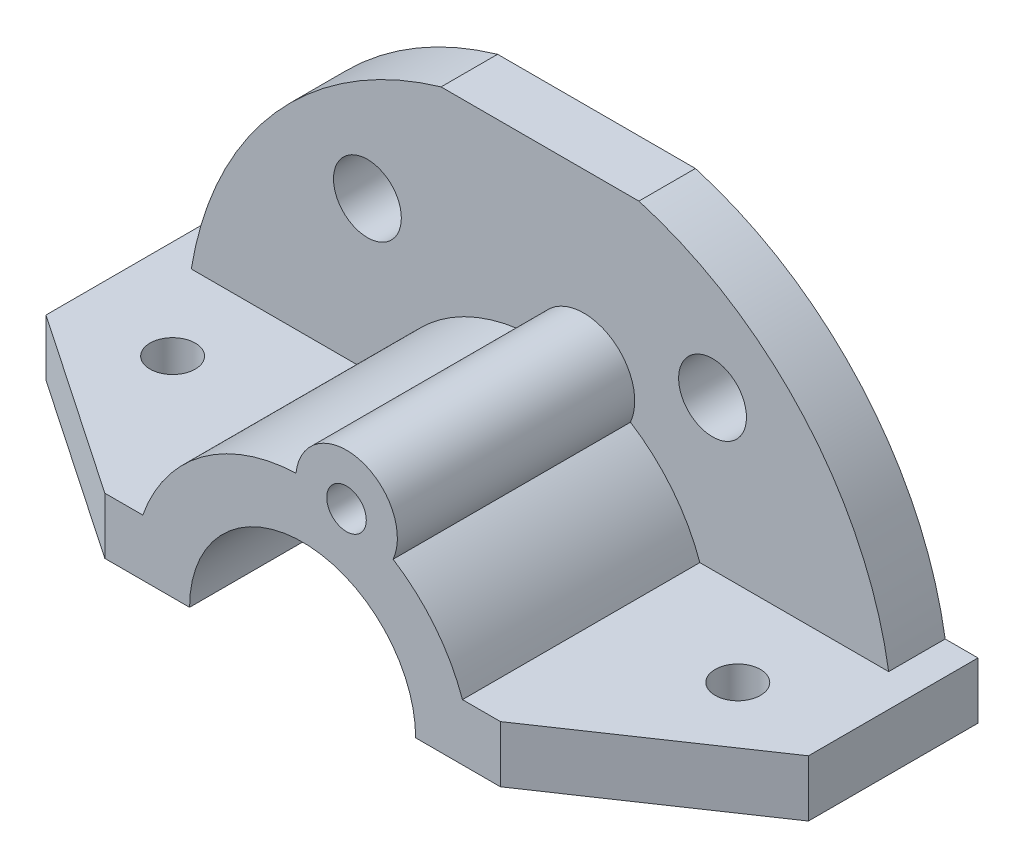
ISO-10303-21;
HEADER;
FILE_DESCRIPTION(('STEP AP214'),'2;1');
FILE_NAME('part.step','',(''),(''),'','','');
FILE_SCHEMA(('AUTOMOTIVE_DESIGN { 1 0 10303 214 1 1 1 1 }'));
ENDSEC;
DATA;
#1=APPLICATION_CONTEXT('core data for automotive mechanical design processes');
#2=APPLICATION_PROTOCOL_DEFINITION('international standard','automotive_design',2000,#1);
#3=PRODUCT_CONTEXT('',#1,'mechanical');
#4=PRODUCT('Part','Part','',(#3));
#5=PRODUCT_RELATED_PRODUCT_CATEGORY('part','',(#4));
#6=PRODUCT_DEFINITION_FORMATION('','',#4);
#7=PRODUCT_DEFINITION_CONTEXT('part definition',#1,'design');
#8=PRODUCT_DEFINITION('design','',#6,#7);
#9=PRODUCT_DEFINITION_SHAPE('','',#8);
#10=(LENGTH_UNIT() NAMED_UNIT(*) SI_UNIT(.MILLI.,.METRE.));
#11=(NAMED_UNIT(*) PLANE_ANGLE_UNIT() SI_UNIT($,.RADIAN.));
#12=(NAMED_UNIT(*) SI_UNIT($,.STERADIAN.) SOLID_ANGLE_UNIT());
#13=UNCERTAINTY_MEASURE_WITH_UNIT(LENGTH_MEASURE(1.E-05),#10,'distance_accuracy_value','');
#14=(GEOMETRIC_REPRESENTATION_CONTEXT(3) GLOBAL_UNCERTAINTY_ASSIGNED_CONTEXT((#13)) GLOBAL_UNIT_ASSIGNED_CONTEXT((#10,
#11,#12)) REPRESENTATION_CONTEXT('',''));
#15=CARTESIAN_POINT('',(0.,0.,0.));
#16=DIRECTION('',(0.,0.,1.));
#17=DIRECTION('',(1.,0.,0.));
#18=AXIS2_PLACEMENT_3D('',#15,#16,#17);
#19=CARTESIAN_POINT('',(0.,0.,52.));
#20=DIRECTION('',(0.,0.,-1.));
#21=DIRECTION('',(-1.,0.,0.));
#22=AXIS2_PLACEMENT_3D('',#19,#20,#21);
#23=CYLINDRICAL_SURFACE('',#22,30.);
#24=CARTESIAN_POINT('',(0.,0.,10.));
#25=DIRECTION('',(0.,0.,1.));
#26=DIRECTION('',(1.,0.,0.));
#27=AXIS2_PLACEMENT_3D('',#24,#25,#26);
#28=CIRCLE('',#27,30.);
#29=CARTESIAN_POINT('',(28.2842712474618,10.0000000000002,10.));
#30=VERTEX_POINT('',#29);
#31=CARTESIAN_POINT('',(16.0101416866023,25.370758033116,10.));
#32=VERTEX_POINT('',#31);
#33=EDGE_CURVE('E176',#30,#32,#28,.T.);
#34=ORIENTED_EDGE('',*,*,#33,.T.);
#35=DIRECTION('',(0.,0.,1.));
#36=VECTOR('',#35,1.);
#37=CARTESIAN_POINT('',(16.0101416866023,25.370758033116,27.));
#38=LINE('',#37,#36);
#39=CARTESIAN_POINT('',(16.0101416866023,25.370758033116,52.));
#40=VERTEX_POINT('',#39);
#41=EDGE_CURVE('E11',#32,#40,#38,.T.);
#42=ORIENTED_EDGE('',*,*,#41,.T.);
#43=CARTESIAN_POINT('',(0.,0.,52.));
#44=DIRECTION('',(0.,0.,1.));
#45=DIRECTION('',(1.,0.,0.));
#46=AXIS2_PLACEMENT_3D('',#43,#44,#45);
#47=CIRCLE('',#46,30.);
#48=CARTESIAN_POINT('',(28.2842712474618,10.0000000000002,52.));
#49=VERTEX_POINT('',#48);
#50=EDGE_CURVE('E172',#49,#40,#47,.T.);
#51=ORIENTED_EDGE('',*,*,#50,.F.);
#52=DIRECTION('',(0.,0.,-1.));
#53=VECTOR('',#52,1.);
#54=CARTESIAN_POINT('',(28.2842712474618,10.0000000000002,52.));
#55=LINE('',#54,#53);
#56=EDGE_CURVE('E202',#49,#30,#55,.T.);
#57=ORIENTED_EDGE('',*,*,#56,.T.);
#58=EDGE_LOOP('',(#34,#42,#51,#57));
#59=FACE_BOUND('',#58,.T.);
#60=ADVANCED_FACE('F43',(#59),#23,.T.);
#61=CARTESIAN_POINT('',(0.,0.,10.));
#62=DIRECTION('',(0.,1.,0.));
#63=DIRECTION('',(-1.,0.,0.));
#64=AXIS2_PLACEMENT_3D('',#61,#62,#63);
#65=PLANE('',#64);
#66=CARTESIAN_POINT('',(-50.,-1.73472347597681E-13,25.));
#67=DIRECTION('',(0.,1.,0.));
#68=DIRECTION('',(-1.,0.,0.));
#69=AXIS2_PLACEMENT_3D('',#66,#67,#68);
#70=CIRCLE('',#69,4.00000000000001);
#71=CARTESIAN_POINT('',(-54.,-1.87438272953053E-13,25.));
#72=VERTEX_POINT('',#71);
#73=EDGE_CURVE('E328',#72,#72,#70,.T.);
#74=ORIENTED_EDGE('',*,*,#73,.T.);
#75=EDGE_LOOP('',(#74));
#76=FACE_BOUND('',#75,.T.);
#77=DIRECTION('',(0.826972369841966,0.,0.562242562883638));
#78=VECTOR('',#77,1.);
#79=CARTESIAN_POINT('',(-35.2419558451316,2.18575157973078E-13,51.8354988879526));
#80=LINE('',#79,#78);
#81=CARTESIAN_POINT('',(-67.5,2.18575157973078E-13,29.9038768886436));
#82=VERTEX_POINT('',#81);
#83=CARTESIAN_POINT('',(-35.,2.18575157973078E-13,52.));
#84=VERTEX_POINT('',#83);
#85=EDGE_CURVE('E265',#82,#84,#80,.T.);
#86=ORIENTED_EDGE('',*,*,#85,.F.);
#87=DIRECTION('',(0.,0.,1.));
#88=VECTOR('',#87,1.);
#89=CARTESIAN_POINT('',(-67.5,2.18575157973078E-13,52.));
#90=LINE('',#89,#88);
#91=CARTESIAN_POINT('',(-67.5,2.18575157973078E-13,-0.0961231113559209));
#92=VERTEX_POINT('',#91);
#93=EDGE_CURVE('E303',#92,#82,#90,.T.);
#94=ORIENTED_EDGE('',*,*,#93,.F.);
#95=DIRECTION('',(-0.999880138885791,0.,-0.015482501791758));
#96=VECTOR('',#95,1.);
#97=CARTESIAN_POINT('',(-67.5,2.18575157973078E-13,-0.0961231113559209));
#98=LINE('',#97,#96);
#99=CARTESIAN_POINT('',(-61.6948133962651,2.18575157973078E-13,-0.00623352509614107));
#100=VERTEX_POINT('',#99);
#101=EDGE_CURVE('E296',#100,#92,#98,.T.);
#102=ORIENTED_EDGE('',*,*,#101,.F.);
#103=DIRECTION('',(0.,0.,-1.));
#104=VECTOR('',#103,1.);
#105=CARTESIAN_POINT('',(-61.6948133962651,2.18575157973078E-13,-0.00623352509614107));
#106=LINE('',#105,#104);
#107=CARTESIAN_POINT('',(-61.6948133962651,-2.15406289676469E-13,0.));
#108=VERTEX_POINT('',#107);
#109=EDGE_CURVE('E315',#108,#100,#106,.T.);
#110=ORIENTED_EDGE('',*,*,#109,.F.);
#111=DIRECTION('',(1.,0.,0.));
#112=VECTOR('',#111,1.);
#113=CARTESIAN_POINT('',(0.,0.,0.));
#114=LINE('',#113,#112);
#115=CARTESIAN_POINT('',(-20.,0.,0.));
#116=VERTEX_POINT('',#115);
#117=EDGE_CURVE('E216',#108,#116,#114,.T.);
#118=ORIENTED_EDGE('',*,*,#117,.T.);
#119=DIRECTION('',(0.,0.,1.));
#120=VECTOR('',#119,1.);
#121=CARTESIAN_POINT('',(-20.,0.,-125.));
#122=LINE('',#121,#120);
#123=CARTESIAN_POINT('',(-20.,0.,52.));
#124=VERTEX_POINT('',#123);
#125=EDGE_CURVE('E200',#116,#124,#122,.T.);
#126=ORIENTED_EDGE('',*,*,#125,.T.);
#127=DIRECTION('',(1.,0.,0.));
#128=VECTOR('',#127,1.);
#129=CARTESIAN_POINT('',(0.,0.,52.));
#130=LINE('',#129,#128);
#131=EDGE_CURVE('E188',#84,#124,#130,.T.);
#132=ORIENTED_EDGE('',*,*,#131,.F.);
#133=EDGE_LOOP('',(#86,#94,#102,#110,#118,#126,#132));
#134=FACE_BOUND('',#133,.T.);
#135=ADVANCED_FACE('F44',(#76,#134),#65,.F.);
#136=CARTESIAN_POINT('',(50.,1.73472347597681E-13,25.));
#137=DIRECTION('',(0.,1.,0.));
#138=DIRECTION('',(-1.,0.,0.));
#139=AXIS2_PLACEMENT_3D('',#136,#137,#138);
#140=CIRCLE('',#139,4.00000000000001);
#141=CARTESIAN_POINT('',(46.,1.59506422242308E-13,25.));
#142=VERTEX_POINT('',#141);
#143=EDGE_CURVE('E316',#142,#142,#140,.T.);
#144=ORIENTED_EDGE('',*,*,#143,.T.);
#145=EDGE_LOOP('',(#144));
#146=FACE_BOUND('',#145,.T.);
#147=DIRECTION('',(0.828109472135937,0.,-0.560566411907403));
#148=VECTOR('',#147,1.);
#149=CARTESIAN_POINT('',(35.1371530595682,2.18575157973078E-13,51.9071579289076));
#150=LINE('',#149,#148);
#151=CARTESIAN_POINT('',(35.,2.18575157973078E-13,52.));
#152=VERTEX_POINT('',#151);
#153=CARTESIAN_POINT('',(67.5,2.18575157973078E-13,30.));
#154=VERTEX_POINT('',#153);
#155=EDGE_CURVE('E70',#152,#154,#150,.T.);
#156=ORIENTED_EDGE('',*,*,#155,.F.);
#157=CARTESIAN_POINT('',(20.,0.,52.));
#158=VERTEX_POINT('',#157);
#159=EDGE_CURVE('E184',#158,#152,#130,.T.);
#160=ORIENTED_EDGE('',*,*,#159,.F.);
#161=DIRECTION('',(0.,0.,1.));
#162=VECTOR('',#161,1.);
#163=CARTESIAN_POINT('',(20.,0.,-125.));
#164=LINE('',#163,#162);
#165=CARTESIAN_POINT('',(20.,0.,0.));
#166=VERTEX_POINT('',#165);
#167=EDGE_CURVE('E271',#158,#166,#164,.F.);
#168=ORIENTED_EDGE('',*,*,#167,.T.);
#169=CARTESIAN_POINT('',(67.5,2.18575157973078E-13,0.));
#170=VERTEX_POINT('',#169);
#171=EDGE_CURVE('E204',#166,#170,#114,.T.);
#172=ORIENTED_EDGE('',*,*,#171,.T.);
#173=DIRECTION('',(0.,0.,-1.));
#174=VECTOR('',#173,1.);
#175=CARTESIAN_POINT('',(67.5,2.18575157973078E-13,52.));
#176=LINE('',#175,#174);
#177=EDGE_CURVE('E283',#154,#170,#176,.T.);
#178=ORIENTED_EDGE('',*,*,#177,.F.);
#179=EDGE_LOOP('',(#156,#160,#168,#172,#178));
#180=FACE_BOUND('',#179,.T.);
#181=ADVANCED_FACE('F367',(#146,#180),#65,.F.);
#182=CARTESIAN_POINT('',(0.,10.0000000000002,52.));
#183=DIRECTION('',(0.,-1.,0.));
#184=DIRECTION('',(0.,0.,-1.));
#185=AXIS2_PLACEMENT_3D('',#182,#183,#184);
#186=PLANE('',#185);
#187=CARTESIAN_POINT('',(50.,10.0000000000002,25.));
#188=DIRECTION('',(0.,1.,0.));
#189=DIRECTION('',(0.,0.,1.));
#190=AXIS2_PLACEMENT_3D('',#187,#188,#189);
#191=CIRCLE('',#190,4.00000000000001);
#192=CARTESIAN_POINT('',(50.,10.0000000000002,29.));
#193=VERTEX_POINT('',#192);
#194=EDGE_CURVE('E335',#193,#193,#191,.T.);
#195=ORIENTED_EDGE('',*,*,#194,.F.);
#196=EDGE_LOOP('',(#195));
#197=FACE_BOUND('',#196,.T.);
#198=DIRECTION('',(0.828109472135937,0.,-0.560566411907403));
#199=VECTOR('',#198,1.);
#200=CARTESIAN_POINT('',(35.1371530595682,10.0000000000002,51.9071579289076));
#201=LINE('',#200,#199);
#202=CARTESIAN_POINT('',(35.,10.0000000000002,52.));
#203=VERTEX_POINT('',#202);
#204=CARTESIAN_POINT('',(67.5,10.0000000000002,30.));
#205=VERTEX_POINT('',#204);
#206=EDGE_CURVE('E320',#203,#205,#201,.T.);
#207=ORIENTED_EDGE('',*,*,#206,.T.);
#208=DIRECTION('',(0.,0.,-1.));
#209=VECTOR('',#208,1.);
#210=CARTESIAN_POINT('',(67.5,10.0000000000002,52.));
#211=LINE('',#210,#209);
#212=CARTESIAN_POINT('',(67.5,10.0000000000002,0.));
#213=VERTEX_POINT('',#212);
#214=EDGE_CURVE('E288',#205,#213,#211,.T.);
#215=ORIENTED_EDGE('',*,*,#214,.T.);
#216=DIRECTION('',(-1.,0.,0.));
#217=VECTOR('',#216,1.);
#218=CARTESIAN_POINT('',(61.6948133962653,10.0000000000002,0.));
#219=LINE('',#218,#217);
#220=CARTESIAN_POINT('',(61.6948133962653,10.0000000000002,0.));
#221=VERTEX_POINT('',#220);
#222=EDGE_CURVE('E290',#213,#221,#219,.T.);
#223=ORIENTED_EDGE('',*,*,#222,.T.);
#224=DIRECTION('',(0.,0.,1.));
#225=VECTOR('',#224,1.);
#226=CARTESIAN_POINT('',(61.6948133962653,10.0000000000002,52.));
#227=LINE('',#226,#225);
#228=CARTESIAN_POINT('',(61.6948133962653,10.0000000000002,10.));
#229=VERTEX_POINT('',#228);
#230=EDGE_CURVE('E284',#221,#229,#227,.T.);
#231=ORIENTED_EDGE('',*,*,#230,.T.);
#232=DIRECTION('',(-1.,0.,0.));
#233=VECTOR('',#232,1.);
#234=CARTESIAN_POINT('',(0.,10.0000000000002,10.));
#235=LINE('',#234,#233);
#236=EDGE_CURVE('E194',#229,#30,#235,.T.);
#237=ORIENTED_EDGE('',*,*,#236,.T.);
#238=ORIENTED_EDGE('',*,*,#56,.F.);
#239=DIRECTION('',(-1.,0.,0.));
#240=VECTOR('',#239,1.);
#241=CARTESIAN_POINT('',(0.,10.0000000000002,52.));
#242=LINE('',#241,#240);
#243=EDGE_CURVE('E179',#203,#49,#242,.T.);
#244=ORIENTED_EDGE('',*,*,#243,.F.);
#245=EDGE_LOOP('',(#207,#215,#223,#231,#237,#238,#244));
#246=FACE_BOUND('',#245,.T.);
#247=ADVANCED_FACE('F407',(#197,#246),#186,.F.);
#248=CARTESIAN_POINT('',(0.,10.0000000000002,52.));
#249=DIRECTION('',(0.,-1.,0.));
#250=DIRECTION('',(0.,0.,-1.));
#251=AXIS2_PLACEMENT_3D('',#248,#249,#250);
#252=PLANE('',#251);
#253=CARTESIAN_POINT('',(-50.,10.0000000000002,25.));
#254=DIRECTION('',(0.,1.,0.));
#255=DIRECTION('',(0.,0.,-1.));
#256=AXIS2_PLACEMENT_3D('',#253,#254,#255);
#257=CIRCLE('',#256,4.00000000000001);
#258=CARTESIAN_POINT('',(-50.,10.0000000000002,21.));
#259=VERTEX_POINT('',#258);
#260=EDGE_CURVE('E236',#259,#259,#257,.T.);
#261=ORIENTED_EDGE('',*,*,#260,.F.);
#262=EDGE_LOOP('',(#261));
#263=FACE_BOUND('',#262,.T.);
#264=DIRECTION('',(0.826972369841966,0.,0.562242562883638));
#265=VECTOR('',#264,1.);
#266=CARTESIAN_POINT('',(-35.2419558451316,10.0000000000002,51.8354988879526));
#267=LINE('',#266,#265);
#268=CARTESIAN_POINT('',(-67.5,10.0000000000002,29.9038768886436));
#269=VERTEX_POINT('',#268);
#270=CARTESIAN_POINT('',(-35.,10.0000000000002,52.));
#271=VERTEX_POINT('',#270);
#272=EDGE_CURVE('E251',#269,#271,#267,.T.);
#273=ORIENTED_EDGE('',*,*,#272,.T.);
#274=DIRECTION('',(-1.,0.,0.));
#275=VECTOR('',#274,1.);
#276=CARTESIAN_POINT('',(0.,10.0000000000002,52.));
#277=LINE('',#276,#275);
#278=CARTESIAN_POINT('',(-28.2842712474618,10.0000000000002,52.));
#279=VERTEX_POINT('',#278);
#280=EDGE_CURVE('E181',#279,#271,#277,.T.);
#281=ORIENTED_EDGE('',*,*,#280,.F.);
#282=DIRECTION('',(0.,0.,-1.));
#283=VECTOR('',#282,1.);
#284=CARTESIAN_POINT('',(-28.2842712474618,10.0000000000002,52.));
#285=LINE('',#284,#283);
#286=CARTESIAN_POINT('',(-28.2842712474618,10.0000000000002,10.));
#287=VERTEX_POINT('',#286);
#288=EDGE_CURVE('E195',#279,#287,#285,.T.);
#289=ORIENTED_EDGE('',*,*,#288,.T.);
#290=DIRECTION('',(-1.,0.,0.));
#291=VECTOR('',#290,1.);
#292=CARTESIAN_POINT('',(0.,10.0000000000002,10.));
#293=LINE('',#292,#291);
#294=CARTESIAN_POINT('',(-61.6948133962651,10.0000000000002,10.));
#295=VERTEX_POINT('',#294);
#296=EDGE_CURVE('E198',#287,#295,#293,.T.);
#297=ORIENTED_EDGE('',*,*,#296,.T.);
#298=DIRECTION('',(0.,0.,-1.));
#299=VECTOR('',#298,1.);
#300=CARTESIAN_POINT('',(-61.6948133962651,10.0000000000002,-0.00623352509614107));
#301=LINE('',#300,#299);
#302=CARTESIAN_POINT('',(-61.6948133962653,10.0000000000002,0.));
#303=VERTEX_POINT('',#302);
#304=EDGE_CURVE('E302',#295,#303,#301,.T.);
#305=ORIENTED_EDGE('',*,*,#304,.T.);
#306=CARTESIAN_POINT('',(-61.6948133962651,10.0000000000002,-0.00623352509614107));
#307=VERTEX_POINT('',#306);
#308=EDGE_CURVE('E304',#303,#307,#301,.T.);
#309=ORIENTED_EDGE('',*,*,#308,.T.);
#310=DIRECTION('',(-0.999880138885791,0.,-0.015482501791758));
#311=VECTOR('',#310,1.);
#312=CARTESIAN_POINT('',(-67.5,10.0000000000002,-0.0961231113559209));
#313=LINE('',#312,#311);
#314=CARTESIAN_POINT('',(-67.5,10.0000000000002,-0.0961231113559209));
#315=VERTEX_POINT('',#314);
#316=EDGE_CURVE('E297',#307,#315,#313,.T.);
#317=ORIENTED_EDGE('',*,*,#316,.T.);
#318=DIRECTION('',(0.,0.,1.));
#319=VECTOR('',#318,1.);
#320=CARTESIAN_POINT('',(-67.5,10.0000000000002,52.));
#321=LINE('',#320,#319);
#322=EDGE_CURVE('E310',#315,#269,#321,.T.);
#323=ORIENTED_EDGE('',*,*,#322,.T.);
#324=EDGE_LOOP('',(#273,#281,#289,#297,#305,#309,#317,#323));
#325=FACE_BOUND('',#324,.T.);
#326=ADVANCED_FACE('F255',(#263,#325),#252,.F.);
#327=CARTESIAN_POINT('',(0.,0.,52.));
#328=DIRECTION('',(0.,0.,1.));
#329=DIRECTION('',(1.,0.,0.));
#330=AXIS2_PLACEMENT_3D('',#327,#328,#329);
#331=PLANE('',#330);
#332=CARTESIAN_POINT('',(7.76457135307553,28.9777747886721,52.));
#333=DIRECTION('',(0.,0.,1.));
#334=DIRECTION('',(1.,0.,0.));
#335=AXIS2_PLACEMENT_3D('',#332,#333,#334);
#336=CIRCLE('',#335,3.5);
#337=CARTESIAN_POINT('',(11.2645713530755,28.9777747886721,52.));
#338=VERTEX_POINT('',#337);
#339=EDGE_CURVE('E344',#338,#338,#336,.T.);
#340=ORIENTED_EDGE('',*,*,#339,.F.);
#341=EDGE_LOOP('',(#340));
#342=FACE_BOUND('',#341,.T.);
#343=ORIENTED_EDGE('',*,*,#50,.T.);
#344=CARTESIAN_POINT('',(7.76457135307553,28.9777747886721,52.));
#345=DIRECTION('',(0.,0.,1.));
#346=DIRECTION('',(1.,0.,0.));
#347=AXIS2_PLACEMENT_3D('',#344,#345,#346);
#348=CIRCLE('',#347,9.);
#349=CARTESIAN_POINT('',(-1.17981040222808,29.9767918132477,52.));
#350=VERTEX_POINT('',#349);
#351=EDGE_CURVE('E56',#40,#350,#348,.T.);
#352=ORIENTED_EDGE('',*,*,#351,.T.);
#353=EDGE_CURVE('E185',#350,#279,#47,.T.);
#354=ORIENTED_EDGE('',*,*,#353,.T.);
#355=ORIENTED_EDGE('',*,*,#280,.T.);
#356=DIRECTION('',(0.,1.,0.));
#357=VECTOR('',#356,1.);
#358=CARTESIAN_POINT('',(-35.,2.18575157973078E-13,52.));
#359=LINE('',#358,#357);
#360=EDGE_CURVE('E257',#84,#271,#359,.T.);
#361=ORIENTED_EDGE('',*,*,#360,.F.);
#362=ORIENTED_EDGE('',*,*,#131,.T.);
#363=CARTESIAN_POINT('',(0.,0.,52.));
#364=DIRECTION('',(0.,0.,1.));
#365=DIRECTION('',(1.,0.,0.));
#366=AXIS2_PLACEMENT_3D('',#363,#364,#365);
#367=CIRCLE('',#366,20.);
#368=EDGE_CURVE('E276',#158,#124,#367,.T.);
#369=ORIENTED_EDGE('',*,*,#368,.F.);
#370=ORIENTED_EDGE('',*,*,#159,.T.);
#371=DIRECTION('',(0.,1.,0.));
#372=VECTOR('',#371,1.);
#373=CARTESIAN_POINT('',(35.,2.18575157973078E-13,52.));
#374=LINE('',#373,#372);
#375=EDGE_CURVE('E322',#152,#203,#374,.T.);
#376=ORIENTED_EDGE('',*,*,#375,.T.);
#377=ORIENTED_EDGE('',*,*,#243,.T.);
#378=EDGE_LOOP('',(#343,#352,#354,#355,#361,#362,#369,#370,#376,#377));
#379=FACE_BOUND('',#378,.T.);
#380=ADVANCED_FACE('F180',(#342,#379),#331,.T.);
#381=CARTESIAN_POINT('',(67.5,2.18575157973078E-13,52.));
#382=DIRECTION('',(1.,0.,0.));
#383=DIRECTION('',(0.,0.,-1.));
#384=AXIS2_PLACEMENT_3D('',#381,#382,#383);
#385=PLANE('',#384);
#386=ORIENTED_EDGE('',*,*,#214,.F.);
#387=DIRECTION('',(0.,1.,0.));
#388=VECTOR('',#387,1.);
#389=CARTESIAN_POINT('',(67.5,2.18575157973078E-13,30.));
#390=LINE('',#389,#388);
#391=EDGE_CURVE('E307',#154,#205,#390,.T.);
#392=ORIENTED_EDGE('',*,*,#391,.F.);
#393=ORIENTED_EDGE('',*,*,#177,.T.);
#394=DIRECTION('',(0.,1.,0.));
#395=VECTOR('',#394,1.);
#396=CARTESIAN_POINT('',(67.5,2.18575157973078E-13,0.));
#397=LINE('',#396,#395);
#398=EDGE_CURVE('E281',#170,#213,#397,.T.);
#399=ORIENTED_EDGE('',*,*,#398,.T.);
#400=EDGE_LOOP('',(#386,#392,#393,#399));
#401=FACE_BOUND('',#400,.T.);
#402=ADVANCED_FACE('F412',(#401),#385,.T.);
#403=CARTESIAN_POINT('',(-67.5,2.18575157973078E-13,52.));
#404=DIRECTION('',(-1.,0.,0.));
#405=DIRECTION('',(0.,0.,1.));
#406=AXIS2_PLACEMENT_3D('',#403,#404,#405);
#407=PLANE('',#406);
#408=ORIENTED_EDGE('',*,*,#93,.T.);
#409=DIRECTION('',(0.,1.,0.));
#410=VECTOR('',#409,1.);
#411=CARTESIAN_POINT('',(-67.5,2.18575157973078E-13,29.9038768886436));
#412=LINE('',#411,#410);
#413=EDGE_CURVE('E261',#82,#269,#412,.T.);
#414=ORIENTED_EDGE('',*,*,#413,.T.);
#415=ORIENTED_EDGE('',*,*,#322,.F.);
#416=DIRECTION('',(0.,1.,0.));
#417=VECTOR('',#416,1.);
#418=CARTESIAN_POINT('',(-67.5,2.18575157973078E-13,-0.0961231113559209));
#419=LINE('',#418,#417);
#420=EDGE_CURVE('E295',#92,#315,#419,.T.);
#421=ORIENTED_EDGE('',*,*,#420,.F.);
#422=EDGE_LOOP('',(#408,#414,#415,#421));
#423=FACE_BOUND('',#422,.T.);
#424=ADVANCED_FACE('F391',(#423),#407,.T.);
#425=CARTESIAN_POINT('',(0.,0.,10.));
#426=DIRECTION('',(0.,0.,-1.));
#427=DIRECTION('',(-1.,0.,0.));
#428=AXIS2_PLACEMENT_3D('',#425,#426,#427);
#429=CYLINDRICAL_SURFACE('',#428,62.5);
#430=ORIENTED_EDGE('',*,*,#304,.F.);
#431=CARTESIAN_POINT('',(0.,0.,10.));
#432=DIRECTION('',(0.,0.,1.));
#433=DIRECTION('',(1.,0.,0.));
#434=AXIS2_PLACEMENT_3D('',#431,#432,#433);
#435=CIRCLE('',#434,62.5);
#436=CARTESIAN_POINT('',(-17.5,60.,10.));
#437=VERTEX_POINT('',#436);
#438=EDGE_CURVE('E215',#437,#295,#435,.T.);
#439=ORIENTED_EDGE('',*,*,#438,.F.);
#440=DIRECTION('',(0.,0.,-1.));
#441=VECTOR('',#440,1.);
#442=CARTESIAN_POINT('',(-17.5,60.,10.));
#443=LINE('',#442,#441);
#444=CARTESIAN_POINT('',(-17.5,60.,0.));
#445=VERTEX_POINT('',#444);
#446=EDGE_CURVE('E213',#437,#445,#443,.T.);
#447=ORIENTED_EDGE('',*,*,#446,.T.);
#448=CARTESIAN_POINT('',(0.,0.,0.));
#449=DIRECTION('',(0.,0.,1.));
#450=DIRECTION('',(1.,0.,0.));
#451=AXIS2_PLACEMENT_3D('',#448,#449,#450);
#452=CIRCLE('',#451,62.5);
#453=EDGE_CURVE('E209',#445,#303,#452,.T.);
#454=ORIENTED_EDGE('',*,*,#453,.T.);
#455=EDGE_LOOP('',(#430,#439,#447,#454));
#456=FACE_BOUND('',#455,.T.);
#457=ADVANCED_FACE('F390',(#456),#429,.T.);
#458=CARTESIAN_POINT('',(0.,0.,10.));
#459=DIRECTION('',(0.,0.,-1.));
#460=DIRECTION('',(-1.,0.,0.));
#461=AXIS2_PLACEMENT_3D('',#458,#459,#460);
#462=CYLINDRICAL_SURFACE('',#461,62.5);
#463=CARTESIAN_POINT('',(0.,0.,10.));
#464=DIRECTION('',(0.,0.,1.));
#465=DIRECTION('',(1.,0.,0.));
#466=AXIS2_PLACEMENT_3D('',#463,#464,#465);
#467=CIRCLE('',#466,62.5);
#468=CARTESIAN_POINT('',(17.5,60.,10.));
#469=VERTEX_POINT('',#468);
#470=EDGE_CURVE('E207',#229,#469,#467,.T.);
#471=ORIENTED_EDGE('',*,*,#470,.F.);
#472=ORIENTED_EDGE('',*,*,#230,.F.);
#473=CARTESIAN_POINT('',(0.,0.,0.));
#474=DIRECTION('',(0.,0.,1.));
#475=DIRECTION('',(1.,0.,0.));
#476=AXIS2_PLACEMENT_3D('',#473,#474,#475);
#477=CIRCLE('',#476,62.5);
#478=CARTESIAN_POINT('',(17.5,60.,0.));
#479=VERTEX_POINT('',#478);
#480=EDGE_CURVE('E217',#221,#479,#477,.T.);
#481=ORIENTED_EDGE('',*,*,#480,.T.);
#482=DIRECTION('',(0.,0.,-1.));
#483=VECTOR('',#482,1.);
#484=CARTESIAN_POINT('',(17.5,60.,10.));
#485=LINE('',#484,#483);
#486=EDGE_CURVE('E228',#469,#479,#485,.T.);
#487=ORIENTED_EDGE('',*,*,#486,.F.);
#488=EDGE_LOOP('',(#471,#472,#481,#487));
#489=FACE_BOUND('',#488,.T.);
#490=ADVANCED_FACE('F388',(#489),#462,.T.);
#491=CARTESIAN_POINT('',(0.,60.,10.));
#492=DIRECTION('',(0.,1.,0.));
#493=DIRECTION('',(0.,0.,1.));
#494=AXIS2_PLACEMENT_3D('',#491,#492,#493);
#495=PLANE('',#494);
#496=DIRECTION('',(1.,0.,0.));
#497=VECTOR('',#496,1.);
#498=CARTESIAN_POINT('',(0.,60.,0.));
#499=LINE('',#498,#497);
#500=EDGE_CURVE('E219',#445,#479,#499,.T.);
#501=ORIENTED_EDGE('',*,*,#500,.F.);
#502=ORIENTED_EDGE('',*,*,#446,.F.);
#503=DIRECTION('',(1.,0.,0.));
#504=VECTOR('',#503,1.);
#505=CARTESIAN_POINT('',(0.,60.,10.));
#506=LINE('',#505,#504);
#507=EDGE_CURVE('E206',#437,#469,#506,.T.);
#508=ORIENTED_EDGE('',*,*,#507,.T.);
#509=ORIENTED_EDGE('',*,*,#486,.T.);
#510=EDGE_LOOP('',(#501,#502,#508,#509));
#511=FACE_BOUND('',#510,.T.);
#512=ADVANCED_FACE('F381',(#511),#495,.T.);
#513=CARTESIAN_POINT('',(0.,0.,10.));
#514=DIRECTION('',(0.,0.,1.));
#515=DIRECTION('',(1.,0.,0.));
#516=AXIS2_PLACEMENT_3D('',#513,#514,#515);
#517=PLANE('',#516);
#518=CARTESIAN_POINT('',(7.76457135307553,28.9777747886721,10.));
#519=DIRECTION('',(0.,0.,1.));
#520=DIRECTION('',(1.,0.,0.));
#521=AXIS2_PLACEMENT_3D('',#518,#519,#520);
#522=CIRCLE('',#521,9.);
#523=CARTESIAN_POINT('',(-1.17981040222807,29.9767918132477,10.));
#524=VERTEX_POINT('',#523);
#525=EDGE_CURVE('E166',#32,#524,#522,.T.);
#526=ORIENTED_EDGE('',*,*,#525,.F.);
#527=ORIENTED_EDGE('',*,*,#33,.F.);
#528=ORIENTED_EDGE('',*,*,#236,.F.);
#529=ORIENTED_EDGE('',*,*,#470,.T.);
#530=ORIENTED_EDGE('',*,*,#507,.F.);
#531=ORIENTED_EDGE('',*,*,#438,.T.);
#532=ORIENTED_EDGE('',*,*,#296,.F.);
#533=EDGE_CURVE('E196',#524,#287,#28,.T.);
#534=ORIENTED_EDGE('',*,*,#533,.F.);
#535=EDGE_LOOP('',(#526,#527,#528,#529,#530,#531,#532,#534));
#536=FACE_BOUND('',#535,.T.);
#537=CARTESIAN_POINT('',(30.5324114601105,36.3871110481515,10.));
#538=DIRECTION('',(0.,0.,1.));
#539=DIRECTION('',(1.,0.,0.));
#540=AXIS2_PLACEMENT_3D('',#537,#538,#539);
#541=CIRCLE('',#540,5.99999999999999);
#542=CARTESIAN_POINT('',(36.5324114601105,36.3871110481515,10.));
#543=VERTEX_POINT('',#542);
#544=EDGE_CURVE('E231',#543,#543,#541,.T.);
#545=ORIENTED_EDGE('',*,*,#544,.F.);
#546=EDGE_LOOP('',(#545));
#547=FACE_BOUND('',#546,.T.);
#548=CARTESIAN_POINT('',(-30.5324114601105,36.3871110481515,10.));
#549=DIRECTION('',(0.,0.,1.));
#550=DIRECTION('',(-1.,0.,0.));
#551=AXIS2_PLACEMENT_3D('',#548,#549,#550);
#552=CIRCLE('',#551,5.99999999999999);
#553=CARTESIAN_POINT('',(-36.5324114601105,36.3871110481515,10.));
#554=VERTEX_POINT('',#553);
#555=EDGE_CURVE('E340',#554,#554,#552,.T.);
#556=ORIENTED_EDGE('',*,*,#555,.F.);
#557=EDGE_LOOP('',(#556));
#558=FACE_BOUND('',#557,.T.);
#559=ADVANCED_FACE('F243',(#536,#547,#558),#517,.T.);
#560=CARTESIAN_POINT('',(0.,0.,0.));
#561=DIRECTION('',(0.,0.,1.));
#562=DIRECTION('',(1.,0.,0.));
#563=AXIS2_PLACEMENT_3D('',#560,#561,#562);
#564=PLANE('',#563);
#565=CARTESIAN_POINT('',(7.76457135307553,28.9777747886721,0.));
#566=DIRECTION('',(0.,0.,1.));
#567=DIRECTION('',(1.,0.,0.));
#568=AXIS2_PLACEMENT_3D('',#565,#566,#567);
#569=CIRCLE('',#568,3.5);
#570=CARTESIAN_POINT('',(11.2645713530755,28.9777747886721,0.));
#571=VERTEX_POINT('',#570);
#572=EDGE_CURVE('E50',#571,#571,#569,.T.);
#573=ORIENTED_EDGE('',*,*,#572,.T.);
#574=EDGE_LOOP('',(#573));
#575=FACE_BOUND('',#574,.T.);
#576=CARTESIAN_POINT('',(30.5324114601105,36.3871110481515,0.));
#577=DIRECTION('',(0.,0.,1.));
#578=DIRECTION('',(1.,0.,0.));
#579=AXIS2_PLACEMENT_3D('',#576,#577,#578);
#580=CIRCLE('',#579,5.99999999999999);
#581=CARTESIAN_POINT('',(36.5324114601105,36.3871110481515,0.));
#582=VERTEX_POINT('',#581);
#583=EDGE_CURVE('E235',#582,#582,#580,.T.);
#584=ORIENTED_EDGE('',*,*,#583,.T.);
#585=EDGE_LOOP('',(#584));
#586=FACE_BOUND('',#585,.T.);
#587=CARTESIAN_POINT('',(-30.5324114601105,36.3871110481515,0.));
#588=DIRECTION('',(0.,0.,1.));
#589=DIRECTION('',(1.,0.,0.));
#590=AXIS2_PLACEMENT_3D('',#587,#588,#589);
#591=CIRCLE('',#590,5.99999999999999);
#592=CARTESIAN_POINT('',(-24.5324114601106,36.3871110481515,0.));
#593=VERTEX_POINT('',#592);
#594=EDGE_CURVE('E230',#593,#593,#591,.T.);
#595=ORIENTED_EDGE('',*,*,#594,.T.);
#596=EDGE_LOOP('',(#595));
#597=FACE_BOUND('',#596,.T.);
#598=ORIENTED_EDGE('',*,*,#117,.F.);
#599=DIRECTION('',(0.,1.,0.));
#600=VECTOR('',#599,1.);
#601=CARTESIAN_POINT('',(-61.6948133962651,0.,0.));
#602=LINE('',#601,#600);
#603=EDGE_CURVE('E293',#108,#303,#602,.T.);
#604=ORIENTED_EDGE('',*,*,#603,.T.);
#605=ORIENTED_EDGE('',*,*,#453,.F.);
#606=ORIENTED_EDGE('',*,*,#500,.T.);
#607=ORIENTED_EDGE('',*,*,#480,.F.);
#608=ORIENTED_EDGE('',*,*,#222,.F.);
#609=ORIENTED_EDGE('',*,*,#398,.F.);
#610=ORIENTED_EDGE('',*,*,#171,.F.);
#611=CARTESIAN_POINT('',(0.,0.,0.));
#612=DIRECTION('',(0.,0.,1.));
#613=DIRECTION('',(1.,0.,0.));
#614=AXIS2_PLACEMENT_3D('',#611,#612,#613);
#615=CIRCLE('',#614,20.);
#616=EDGE_CURVE('E273',#166,#116,#615,.T.);
#617=ORIENTED_EDGE('',*,*,#616,.T.);
#618=EDGE_LOOP('',(#598,#604,#605,#606,#607,#608,#609,#610,#617));
#619=FACE_BOUND('',#618,.T.);
#620=ADVANCED_FACE('F349',(#575,#586,#597,#619),#564,.F.);
#621=ORIENTED_EDGE('',*,*,#353,.F.);
#622=DIRECTION('',(0.,0.,1.));
#623=VECTOR('',#622,1.);
#624=CARTESIAN_POINT('',(-1.17981040222808,29.9767918132477,27.));
#625=LINE('',#624,#623);
#626=EDGE_CURVE('E55',#350,#524,#625,.F.);
#627=ORIENTED_EDGE('',*,*,#626,.T.);
#628=ORIENTED_EDGE('',*,*,#533,.T.);
#629=ORIENTED_EDGE('',*,*,#288,.F.);
#630=EDGE_LOOP('',(#621,#627,#628,#629));
#631=FACE_BOUND('',#630,.T.);
#632=ADVANCED_FACE('F237',(#631),#23,.T.);
#633=CARTESIAN_POINT('',(0.,0.,-125.));
#634=DIRECTION('',(0.,0.,1.));
#635=DIRECTION('',(1.,0.,0.));
#636=AXIS2_PLACEMENT_3D('',#633,#634,#635);
#637=CYLINDRICAL_SURFACE('',#636,20.);
#638=ORIENTED_EDGE('',*,*,#616,.F.);
#639=ORIENTED_EDGE('',*,*,#167,.F.);
#640=ORIENTED_EDGE('',*,*,#368,.T.);
#641=ORIENTED_EDGE('',*,*,#125,.F.);
#642=EDGE_LOOP('',(#638,#639,#640,#641));
#643=FACE_BOUND('',#642,.T.);
#644=ADVANCED_FACE('F372',(#643),#637,.F.);
#645=CARTESIAN_POINT('',(-61.6948133962651,2.18575157973078E-13,-0.00623352509614107));
#646=DIRECTION('',(1.,0.,0.));
#647=DIRECTION('',(0.,0.,-1.));
#648=AXIS2_PLACEMENT_3D('',#645,#646,#647);
#649=PLANE('',#648);
#650=ORIENTED_EDGE('',*,*,#603,.F.);
#651=ORIENTED_EDGE('',*,*,#109,.T.);
#652=DIRECTION('',(0.,1.,0.));
#653=VECTOR('',#652,1.);
#654=CARTESIAN_POINT('',(-61.6948133962651,2.18575157973078E-13,-0.00623352509614107));
#655=LINE('',#654,#653);
#656=EDGE_CURVE('E294',#100,#307,#655,.T.);
#657=ORIENTED_EDGE('',*,*,#656,.T.);
#658=ORIENTED_EDGE('',*,*,#308,.F.);
#659=EDGE_LOOP('',(#650,#651,#657,#658));
#660=FACE_BOUND('',#659,.T.);
#661=ADVANCED_FACE('F377',(#660),#649,.T.);
#662=CARTESIAN_POINT('',(-67.5,2.18575157973078E-13,-0.0961231113559209));
#663=DIRECTION('',(0.015482501791758,0.,-0.999880138885791));
#664=DIRECTION('',(-0.999880138885791,0.,-0.015482501791758));
#665=AXIS2_PLACEMENT_3D('',#662,#663,#664);
#666=PLANE('',#665);
#667=ORIENTED_EDGE('',*,*,#316,.F.);
#668=ORIENTED_EDGE('',*,*,#656,.F.);
#669=ORIENTED_EDGE('',*,*,#101,.T.);
#670=ORIENTED_EDGE('',*,*,#420,.T.);
#671=EDGE_LOOP('',(#667,#668,#669,#670));
#672=FACE_BOUND('',#671,.T.);
#673=ADVANCED_FACE('F435',(#672),#666,.T.);
#674=CARTESIAN_POINT('',(-35.2419558451316,2.18575157973078E-13,51.8354988879526));
#675=DIRECTION('',(-0.562242562883638,0.,0.826972369841966));
#676=DIRECTION('',(0.826972369841966,0.,0.562242562883638));
#677=AXIS2_PLACEMENT_3D('',#674,#675,#676);
#678=PLANE('',#677);
#679=ORIENTED_EDGE('',*,*,#272,.F.);
#680=ORIENTED_EDGE('',*,*,#413,.F.);
#681=ORIENTED_EDGE('',*,*,#85,.T.);
#682=ORIENTED_EDGE('',*,*,#360,.T.);
#683=EDGE_LOOP('',(#679,#680,#681,#682));
#684=FACE_BOUND('',#683,.T.);
#685=ADVANCED_FACE('F421',(#684),#678,.T.);
#686=CARTESIAN_POINT('',(35.1371530595682,2.18575157973078E-13,51.9071579289076));
#687=DIRECTION('',(0.560566411907403,0.,0.828109472135937));
#688=DIRECTION('',(0.828109472135937,0.,-0.560566411907403));
#689=AXIS2_PLACEMENT_3D('',#686,#687,#688);
#690=PLANE('',#689);
#691=ORIENTED_EDGE('',*,*,#206,.F.);
#692=ORIENTED_EDGE('',*,*,#375,.F.);
#693=ORIENTED_EDGE('',*,*,#155,.T.);
#694=ORIENTED_EDGE('',*,*,#391,.T.);
#695=EDGE_LOOP('',(#691,#692,#693,#694));
#696=FACE_BOUND('',#695,.T.);
#697=ADVANCED_FACE('F419',(#696),#690,.T.);
#698=CARTESIAN_POINT('',(-50.,-45.9999999999998,25.));
#699=DIRECTION('',(0.,1.,0.));
#700=DIRECTION('',(0.,0.,1.));
#701=AXIS2_PLACEMENT_3D('',#698,#699,#700);
#702=CYLINDRICAL_SURFACE('',#701,4.00000000000001);
#703=ORIENTED_EDGE('',*,*,#260,.T.);
#704=EDGE_LOOP('',(#703));
#705=FACE_BOUND('',#704,.T.);
#706=ORIENTED_EDGE('',*,*,#73,.F.);
#707=EDGE_LOOP('',(#706));
#708=FACE_BOUND('',#707,.T.);
#709=ADVANCED_FACE('F422',(#705,#708),#702,.F.);
#710=CARTESIAN_POINT('',(50.,-45.9999999999998,25.));
#711=DIRECTION('',(0.,1.,0.));
#712=DIRECTION('',(0.,0.,1.));
#713=AXIS2_PLACEMENT_3D('',#710,#711,#712);
#714=CYLINDRICAL_SURFACE('',#713,4.00000000000001);
#715=ORIENTED_EDGE('',*,*,#194,.T.);
#716=EDGE_LOOP('',(#715));
#717=FACE_BOUND('',#716,.T.);
#718=ORIENTED_EDGE('',*,*,#143,.F.);
#719=EDGE_LOOP('',(#718));
#720=FACE_BOUND('',#719,.T.);
#721=ADVANCED_FACE('F429',(#717,#720),#714,.F.);
#722=CARTESIAN_POINT('',(-30.5324114601105,36.3871110481515,-46.));
#723=DIRECTION('',(0.,0.,1.));
#724=DIRECTION('',(1.,0.,0.));
#725=AXIS2_PLACEMENT_3D('',#722,#723,#724);
#726=CYLINDRICAL_SURFACE('',#725,5.99999999999999);
#727=ORIENTED_EDGE('',*,*,#555,.T.);
#728=EDGE_LOOP('',(#727));
#729=FACE_BOUND('',#728,.T.);
#730=ORIENTED_EDGE('',*,*,#594,.F.);
#731=EDGE_LOOP('',(#730));
#732=FACE_BOUND('',#731,.T.);
#733=ADVANCED_FACE('F463',(#729,#732),#726,.F.);
#734=CARTESIAN_POINT('',(30.5324114601105,36.3871110481515,-46.));
#735=DIRECTION('',(0.,0.,1.));
#736=DIRECTION('',(1.,0.,0.));
#737=AXIS2_PLACEMENT_3D('',#734,#735,#736);
#738=CYLINDRICAL_SURFACE('',#737,5.99999999999999);
#739=ORIENTED_EDGE('',*,*,#544,.T.);
#740=EDGE_LOOP('',(#739));
#741=FACE_BOUND('',#740,.T.);
#742=ORIENTED_EDGE('',*,*,#583,.F.);
#743=EDGE_LOOP('',(#742));
#744=FACE_BOUND('',#743,.T.);
#745=ADVANCED_FACE('F359',(#741,#744),#738,.F.);
#746=CARTESIAN_POINT('',(7.76457135307553,28.9777747886721,2.));
#747=DIRECTION('',(0.,0.,1.));
#748=DIRECTION('',(1.,0.,0.));
#749=AXIS2_PLACEMENT_3D('',#746,#747,#748);
#750=CYLINDRICAL_SURFACE('',#749,9.);
#751=ORIENTED_EDGE('',*,*,#41,.F.);
#752=ORIENTED_EDGE('',*,*,#525,.T.);
#753=ORIENTED_EDGE('',*,*,#626,.F.);
#754=ORIENTED_EDGE('',*,*,#351,.F.);
#755=EDGE_LOOP('',(#751,#752,#753,#754));
#756=FACE_BOUND('',#755,.T.);
#757=ADVANCED_FACE('F165',(#756),#750,.T.);
#758=CARTESIAN_POINT('',(7.76457135307553,28.9777747886721,-23.));
#759=DIRECTION('',(0.,0.,1.));
#760=DIRECTION('',(1.,0.,0.));
#761=AXIS2_PLACEMENT_3D('',#758,#759,#760);
#762=CYLINDRICAL_SURFACE('',#761,3.5);
#763=ORIENTED_EDGE('',*,*,#339,.T.);
#764=EDGE_LOOP('',(#763));
#765=FACE_BOUND('',#764,.T.);
#766=ORIENTED_EDGE('',*,*,#572,.F.);
#767=EDGE_LOOP('',(#766));
#768=FACE_BOUND('',#767,.T.);
#769=ADVANCED_FACE('F352',(#765,#768),#762,.F.);
#770=CLOSED_SHELL('',(#60,#135,#181,#247,#326,#380,#402,#424,#457,#490,#512,#559,#620,#632,#644,
#661,#673,#685,#697,#709,#721,#733,#745,#757,#769));
#771=MANIFOLD_SOLID_BREP('B2',#770);
#772=ADVANCED_BREP_SHAPE_REPRESENTATION('',(#18,#771),#14);
#773=SHAPE_DEFINITION_REPRESENTATION(#9,#772);
ENDSEC;
END-ISO-10303-21;
